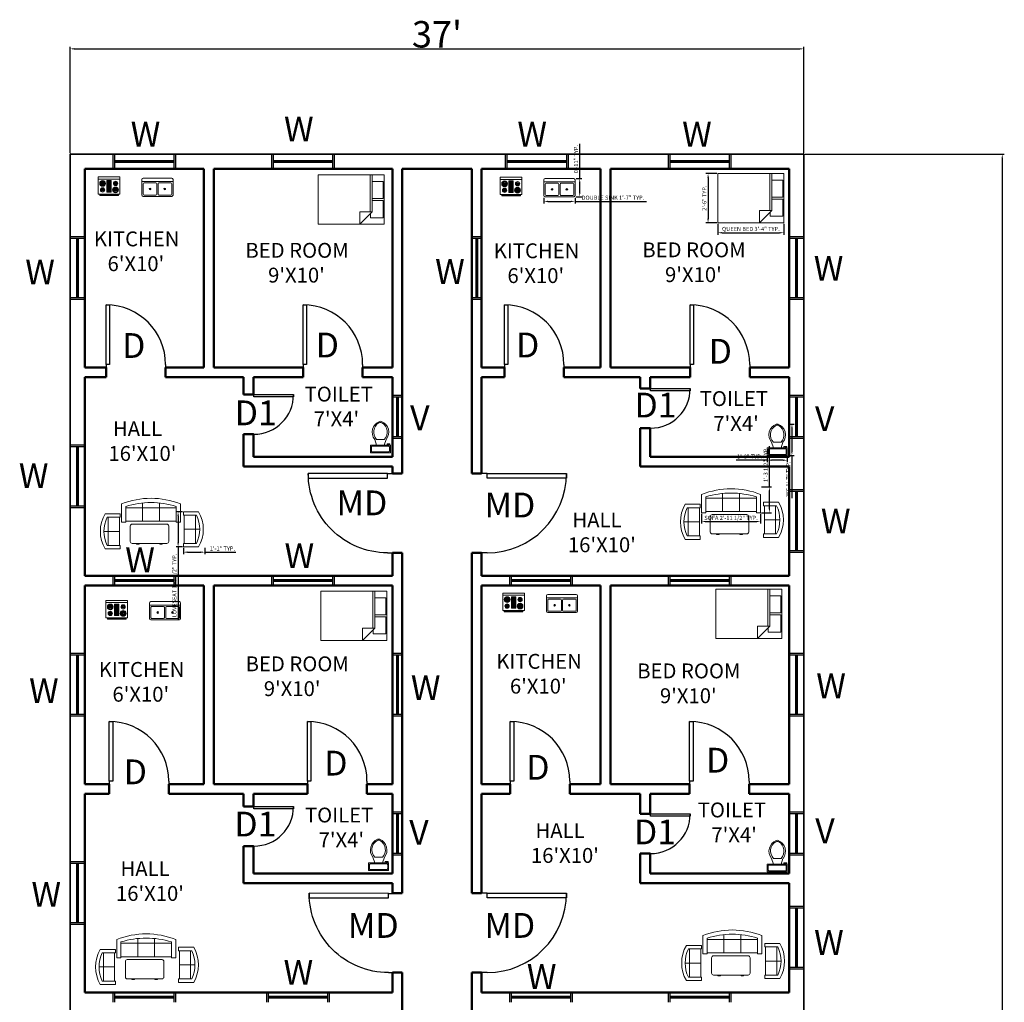
# Model space of a CAD drawing. Units: inches. Extents: x -25308 to -23933, y 10755 to 11996.
# Tile 6 of 6: x -24529 to -23933, y 11402 to 11996. Entities that reach past the tile are written whole.
import ezdxf

# ---------------------------------------------------------------- set-up
doc = ezdxf.new("R2010")
doc.units = ezdxf.units.IN
for name, color, linetype, lineweight in [('A-ANNO-DIMS', 2, 'Continuous', 18), ('A-ANNO-SYMB', 3, 'Continuous', 18), ('A-AREA-IDEN', 7, 'Continuous', 18), ('A-DOOR', 3, 'Continuous', 25), ('A-FLOR-FIXT', 8, 'Continuous', 18), ('A-FURN', 8, 'Continuous', 18), ('A-GLAZ', 4, 'Continuous', 25), ('A-WALL', 7, 'Continuous', 50), ('C-PROP', 30, 'Continuous', 35)]:
    doc.layers.add(name, color=color, linetype=linetype, lineweight=lineweight)
doc.styles.get("Standard").update_dxf_attribs({"font": 'arial.ttf'})
doc.dimstyles.new('ISO-25', dxfattribs={"dimtxt": 2.5, "dimasz": 2.5, "dimexe": 1.25, "dimexo": 0.625, "dimtad": 1, "dimdec": 0, "dimlunit": 3, "dimtxsty": 'Standard', "dimcen": 2.5, "dimadec": 0, "dimazin": 0, "dimtfac": 1, "dimtdec": 0, "dimtmove": 0, "dimatfit": 3, "dimfxl": 1, "dimarcsym": 0})

# ---------------------------------------------------------------- blocks, each defined once
blk = doc.blocks.new('*U8')
for p, q in [((0, 0), (0, -100)), ((750, 0), (750, -100))]:
    blk.add_line(p, q)
blk.add_lwpolyline([(0, 0), (0, 750), (43.75, 750), (43.75, 0)], close=True)
blk.add_arc((0, 0), 750, 0, 90)
blk = doc.blocks.new('Range-Oven - 30 in top')
for p, q in [((0, -3), (30, -3)), ((12, -6), (18, -6)), ((13, -20), (13, -6)), ((14, -6), (14, -20)), ((15, -20), (15, -6)), ((16, -6), (16, -20)), ((17, -20), (17, -6)), ((6, -24), (6, -25)), ((8, -25), (8, -24)), ((18, -20), (12, -20)), ((22, -25), (22, -24)), ((24, -24), (24, -25))]:
    blk.add_line(p, q)
for points in [[(0, -24), (0, 0), (30, 0), (30, -24)], [(12, -21), (12, -5), (18, -5), (18, -21)], [(2, -26), (2, -25), (28, -25), (28, -26)]]:
    blk.add_lwpolyline(points, close=True)
for centre, radius in [((6, -9), 4), ((6, -9), 3), ((6, -9), 2), ((6, -9), 1), ((24, -9), 3), ((24, -9), 2), ((24, -9), 1), ((6, -18), 3), ((6, -18), 2), ((6, -18), 1), ((24, -18), 4), ((24, -18), 3), ((24, -18), 2), ((24, -18), 1)]:
    blk.add_circle(centre, radius)
blk = doc.blocks.new('Sink-double - 36 in top')
for p, q in [((-18, -4), (18, -4)), ((-0.75, -18.5), (-0.75, -6.5)), ((0.75, -6.5), (0.75, -18.5))]:
    blk.add_line(p, q)
for points in [[(-16.5, 0), (16.5, 0)], [(-18, -19.5), (-18, -1.5)], [(-16.5, -18.5), (-16.5, -6.5)], [(-15.5, -5.5), (-1.75, -5.5)], [(1.75, -5.5), (15.5, -5.5)], [(16.5, -6.5), (16.5, -18.5)], [(18, -1.5), (18, -19.5)], [(16.5, -21), (-16.5, -21)], [(-1.75, -19.5), (-15.5, -19.5)], [(15.5, -19.5), (1.75, -19.5)]]:
    blk.add_lwpolyline(points)
for centre, radius in [((-8.5, -12.5), 1), ((-8.5, -12.5), 0.5), ((8.5, -12.5), 1), ((8.5, -12.5), 0.5)]:
    blk.add_circle(centre, radius)
for centre, radius, start, end in [((-16.5, -1.5), 1.5, 90, 180), ((16.5, -1.5), 1.5, 0, 90), ((-15.5, -6.5), 1, 90, 180), ((-1.75, -6.5), 1, 0, 90), ((1.75, -6.5), 1, 90, 180), ((15.5, -6.5), 1, 0, 90), ((-16.5, -19.5), 1.5, 180, 270), ((-15.5, -18.5), 1, 180, 270), ((-1.75, -18.5), 1, 270, 0), ((1.75, -18.5), 1, 180, 270), ((15.5, -18.5), 1, 270, 0), ((16.5, -19.5), 1.5, 270, 0)]:
    blk.add_arc(centre, radius, start, end)
blk = doc.blocks.new('Bed - Queen')
for p, q in [((0, -80.00003), (0, 0)), ((0, 0), (59.99999, 0)), ((59.99999, 0), (59.99999, -80.00003)), ((7.99999, -1.2), (28.79998, -1.2)), ((7.99999, -14.4), (7.99999, -1.2)), ((28.79998, -1.2), (28.79998, -14.4)), ((31.19999, -1.2), (51.99999, -1.2)), ((31.19999, -14.4), (31.19999, -1.2)), ((51.99999, -1.2), (51.99999, -16.4)), ((0, -14.4), (44.8, -14.4)), ((44.8, -16.8), (0, -16.8)), ((59.99999, -29.6), (44.8, -14.4)), ((44.8, -14.4), (44.8, -29.6)), ((51.99999, -16.4), (46.79936, -16.4)), ((44.8, -29.6), (59.99999, -29.6)), ((59.99999, -80.00003), (0, -80.00003))]:
    blk.add_line(p, q)
blk = doc.blocks.new('Desk - 30 x 60 in.')
for p, q in [((-26.999995, 0), (26.999995, 0)), ((-29.999995, -27), (-29.999995, -3)), ((29.999995, -3), (29.999995, -27)), ((26.999995, -30), (-26.999995, -30)), ((-20.000005, -30), (-20.000005, -31)), ((-16.000005, -31), (-16.000005, -30)), ((15.999995, -31), (15.999995, -30)), ((19.999995, -30), (19.999995, -31)), ((-20.000005, -31), (-16.000005, -31)), ((19.999995, -31), (15.999995, -31))]:
    blk.add_line(p, q)
for centre, start, end in [((-26.499995, -3.5), 98.1301, 171.8699), ((26.499995, -3.5), 8.130102, 81.8699), ((-26.499995, -26.5), 188.1301, 261.8699), ((26.499995, -26.5), 278.1301, 351.8699)]:
    blk.add_arc(centre, 3.535534, start, end)
blk = doc.blocks.new('Sofa - Roundback 7 ft.')
for p, q in [((-36.000027, -34), (-36.000027, -11.4696)), ((-35.999844, -13.3819), (35.9998, -13.3819)), ((-12.00002, -32.4421), (-12.00003, -6.5971)), ((11.99997, -32.4421), (11.99998, -6.5971)), ((35.99998, -34), (35.99998, -11.4696)), ((-36.000027, -32.4421), (35.99998, -32.4421))]:
    blk.add_line(p, q)
for points in [[(-36.000027, -34), (-42.000027, -34), (-42.000027, -8)], [(41.99998, -8), (41.99998, -34), (35.99998, -34)]]:
    blk.add_lwpolyline(points)
for centre, radius, start, end in [((0, -114.25), 114.25, 68.43141, 111.5686), ((-0.00001, -127.1968), 121.1968, 72.72033, 107.2797)]:
    blk.add_arc(centre, radius, start, end)
blk = doc.blocks.new('Sofa - Roundback Loveseat 5 ft.')
for p, q in [((-24, -33.99998), (-24, -11.46958)), ((-23.9998, -13.38178), (23.99986, -13.38178)), ((0, -32.44198), (0, -5.99998)), ((24.00004, -33.99998), (24.00004, -11.46958)), ((-24, -32.44198), (24.00004, -32.44198))]:
    blk.add_line(p, q)
for points in [[(-24, -33.99998), (-30, -33.99998), (-30, -7.99998)], [(30.00004, -7.99998), (30.00004, -33.99998), (24.00004, -33.99998)]]:
    blk.add_lwpolyline(points)
for centre, radius, start, end in [((0, -60.24998), 60.24998, 60.13715, 119.8628), ((0, -61.38438), 55.38444, 64.32083, 115.6792)]:
    blk.add_arc(centre, radius, start, end)
blk = doc.blocks.new('Toilet - top')
for p, q in [((-10, -8.5), (-8, -8.5)), ((-10, -9.5), (-10, -8.5)), ((-7, -9.5), (-10, -9.5)), ((-8, -8.5), (-8, -8)), ((-7, -8), (-7, -9.5)), ((-4, -8), (-6, -14)), ((4, -8), (6, -14)), ((9.5, -6), (9.5, -2)), ((4, -14), (-4, -14))]:
    blk.add_line(p, q)
blk.add_lwpolyline([(10.5, -8), (10.5, 0), (-10.5, 0), (-10.5, -8)], close=True)
for points in [[(-9.5, -2), (-9.5, -6)], [(8.5, -1), (-8.5, -1)], [(-8.5, -7), (8.5, -7)]]:
    blk.add_lwpolyline(points)
for centre, radius, start, end in [((-8.6, -1.9), 0.884, 81.8699, 188.1301), ((-8.6, -6.1), 0.884, 171.8699, 278.1301), ((8.6, -1.9), 0.884, 351.8699, 98.1301), ((8.6, -6.1), 0.884, 261.8699, 8.1301), ((3.5, -21.6), 12.2, 141.4691, 247.9714), ((4.2, -21.8), 11.3, 136.3677, 238.9468), ((-3.5, -21.6), 12.2, 292.0284, 38.5307), ((-4.2, -21.8), 11.3, 301.053, 43.6321), ((0, -27.9), 4, 245.7318, 294.2682), ((0, -29), 4, 254.8605, 285.1395)]:
    blk.add_arc(centre, radius, start, end)
blk = doc.blocks.new('*D172')
at = {"layer": 'A-ANNO-DIMS', "color": 0, "lineweight": -2, "transparency": 16777216}
for p, q in [((-24498.33, 11915.75), (-24498.33, 11980.03)), ((-24054.33, 11915.75), (-24054.33, 11980.03)), ((-24495.83, 11978.78), (-24056.83, 11978.78))]:
    blk.add_line(p, q, dxfattribs=at)
at = {"layer": 'A-ANNO-DIMS', "color": 0, "transparency": 16777216}
for points in [[(-24495.83, 11979.2), (-24495.83, 11978.37), (-24498.33, 11978.78)], [(-24056.83, 11979.2), (-24056.83, 11978.37), (-24054.33, 11978.78)]]:
    blk.add_solid(points, dxfattribs=at)
at = {"layer": 'Defpoints', "color": 0, "transparency": 16777216}
for p in [(-24054.33, 11978.78), (-24498.33, 11915.12), (-24054.33, 11915.12)]:
    blk.add_point(p, dxfattribs=at)
at = {"layer": 'A-ANNO-DIMS', "color": 0, "transparency": 16777216, "insert": (-24276.33, 11987.58), "char_height": 2.5, "attachment_point": 5}
blk.add_mtext("{\\H6.4x;37'}", dxfattribs=at)
blk = doc.blocks.new('*D173')
at = {"layer": 'A-ANNO-DIMS', "color": 0, "lineweight": -2, "transparency": 16777216}
for p, q in [((-24053.71, 11915.12), (-23933.08, 11915.12)), ((-23934.33, 11912.62), (-23934.33, 10813.62)), ((-24053.71, 10811.12), (-23933.08, 10811.12))]:
    blk.add_line(p, q, dxfattribs=at)
at = {"layer": 'A-ANNO-DIMS', "color": 0, "transparency": 16777216}
for points in [[(-23934.75, 11912.62), (-23933.91, 11912.62), (-23934.33, 11915.12)], [(-23934.75, 10813.62), (-23933.91, 10813.62), (-23934.33, 10811.12)]]:
    blk.add_solid(points, dxfattribs=at)
at = {"layer": 'Defpoints', "color": 0, "transparency": 16777216}
for p in [(-24054.33, 11915.12), (-24054.33, 10811.12), (-23934.33, 10811.12)]:
    blk.add_point(p, dxfattribs=at)
at = {"layer": 'A-ANNO-DIMS', "color": 0, "transparency": 16777216, "insert": (-23943.13, 11363.12), "char_height": 2.5, "attachment_point": 5, "rotation": 90}
blk.add_mtext("{\\H6.4x;92'}", dxfattribs=at)
blk = doc.blocks.new('WIN-36-9IN')
for p, q in [((0, 9), (0, 0)), ((1, 9), (1, 0)), ((37, 9), (37, 0)), ((38, 9), (38, 0)), ((1, 5), (37, 5)), ((1, 4.5), (37, 4.5)), ((1, 4), (37, 4))]:
    blk.add_line(p, q)
blk = doc.blocks.new('VENT-24')
for p, q in [((0, 26), (9, 26)), ((0, 25), (9, 25)), ((4, 1), (4, 25)), ((4.5, 1), (4.5, 25)), ((5, 1), (5, 25)), ((0, 1), (9, 1)), ((0, 0), (9, 0))]:
    blk.add_line(p, q)
blk = doc.blocks.new('WIN-24-6IN')
for p, q in [((0, 26), (6, 26)), ((0, 25), (6, 25)), ((2.5, 1), (2.5, 25)), ((3, 1), (3, 25)), ((3.5, 1), (3.5, 25)), ((0, 1), (6, 1)), ((0, 0), (6, 0))]:
    blk.add_line(p, q)
blk = doc.blocks.new('WIN-36-6IN')
for p, q in [((0, 6), (0, 0)), ((1, 6), (1, 0)), ((37, 6), (37, 0)), ((38, 6), (38, 0)), ((1, 3.5), (37, 3.5)), ((1, 3), (37, 3)), ((1, 2.5), (37, 2.5))]:
    blk.add_line(p, q)
blk = doc.blocks.new('*D194')
at = {"layer": 'A-ANNO-DIMS', "color": 0, "lineweight": -2, "transparency": 16777216}
for p, q in [((-24430.39, 11698.82), (-24434.2, 11698.82)), ((-24432.95, 11696.32), (-24432.95, 11680.06)), ((-24430.39, 11677.56), (-24434.2, 11677.56)), ((-24432.95, 11677.56), (-24432.95, 11633.45))]:
    blk.add_line(p, q, dxfattribs=at)
at = {"layer": 'A-ANNO-DIMS', "color": 0, "transparency": 16777216}
for points in [[(-24433.37, 11696.32), (-24432.53, 11696.32), (-24432.95, 11698.82)], [(-24433.37, 11680.06), (-24432.53, 11680.06), (-24432.95, 11677.56)]]:
    blk.add_solid(points, dxfattribs=at)
at = {"layer": 'Defpoints', "color": 0, "transparency": 16777216}
for p in [(-24429.76, 11698.82), (-24432.95, 11677.56), (-24429.76, 11677.56)]:
    blk.add_point(p, dxfattribs=at)
at = {"layer": 'A-ANNO-DIMS', "color": 0, "transparency": 16777216, "insert": (-24434.87, 11654.25), "char_height": 2.5, "attachment_point": 5, "rotation": 90}
blk.add_mtext('LOVESEAT 1\'-9 1/2" TYP.', dxfattribs=at)
blk = doc.blocks.new('*D195')
at = {"layer": 'A-ANNO-DIMS', "color": 0, "lineweight": -2, "transparency": 16777216}
for p, q in [((-24429.76, 11676.94), (-24429.76, 11673.12)), ((-24416.77, 11676.94), (-24416.77, 11673.12)), ((-24427.26, 11674.37), (-24419.27, 11674.37)), ((-24416.77, 11674.37), (-24398.02, 11674.37))]:
    blk.add_line(p, q, dxfattribs=at)
at = {"layer": 'A-ANNO-DIMS', "color": 0, "transparency": 16777216}
for points in [[(-24427.26, 11674.79), (-24427.26, 11673.95), (-24429.76, 11674.37)], [(-24419.27, 11674.79), (-24419.27, 11673.95), (-24416.77, 11674.37)]]:
    blk.add_solid(points, dxfattribs=at)
at = {"layer": 'Defpoints', "color": 0, "transparency": 16777216}
for p in [(-24429.76, 11677.56), (-24416.77, 11677.56), (-24416.77, 11674.37)]:
    blk.add_point(p, dxfattribs=at)
at = {"layer": 'A-ANNO-DIMS', "color": 0, "transparency": 16777216, "insert": (-24406.14, 11676.25), "char_height": 2.5, "attachment_point": 5}
blk.add_mtext('1\'-1" TYP.', dxfattribs=at)
blk = doc.blocks.new('*D200')
at = {"layer": 'A-ANNO-DIMS', "color": 0, "lineweight": -2, "transparency": 16777216}
for p, q in [((-24116.24, 11697.6), (-24116.24, 11691.62)), ((-24080.56, 11697.6), (-24080.56, 11691.62)), ((-24113.74, 11692.87), (-24083.06, 11692.87))]:
    blk.add_line(p, q, dxfattribs=at)
at = {"layer": 'A-ANNO-DIMS', "color": 0, "transparency": 16777216}
for points in [[(-24113.74, 11693.29), (-24113.74, 11692.45), (-24116.24, 11692.87)], [(-24083.06, 11693.29), (-24083.06, 11692.45), (-24080.56, 11692.87)]]:
    blk.add_solid(points, dxfattribs=at)
at = {"layer": 'Defpoints', "color": 0, "transparency": 16777216}
for p in [(-24116.24, 11698.22), (-24080.56, 11698.22), (-24080.56, 11692.87)]:
    blk.add_point(p, dxfattribs=at)
at = {"layer": 'A-ANNO-DIMS', "color": 0, "transparency": 16777216, "insert": (-24098.4, 11694.79), "char_height": 2.5, "attachment_point": 5}
blk.add_mtext('SOFA 2\'-11 1/2" TYP.', dxfattribs=at)
blk = doc.blocks.new('*D201')
at = {"layer": 'A-ANNO-DIMS', "color": 0, "lineweight": -2, "transparency": 16777216}
for p, q in [((-24075.2, 11713.8), (-24075.2, 11738.38)), ((-24079.93, 11713.8), (-24073.95, 11713.8)), ((-24075.2, 11700.72), (-24075.2, 11711.3)), ((-24079.93, 11698.22), (-24073.95, 11698.22))]:
    blk.add_line(p, q, dxfattribs=at)
at = {"layer": 'A-ANNO-DIMS', "color": 0, "transparency": 16777216}
for points in [[(-24075.62, 11711.3), (-24074.79, 11711.3), (-24075.2, 11713.8)], [(-24075.62, 11700.72), (-24074.79, 11700.72), (-24075.2, 11698.22)]]:
    blk.add_solid(points, dxfattribs=at)
at = {"layer": 'Defpoints', "color": 0, "transparency": 16777216}
for p in [(-24080.56, 11713.8), (-24075.2, 11713.8), (-24080.56, 11698.22)]:
    blk.add_point(p, dxfattribs=at)
at = {"layer": 'A-ANNO-DIMS', "color": 0, "transparency": 16777216, "insert": (-24077.12, 11727.34), "char_height": 2.5, "attachment_point": 5, "rotation": 90}
blk.add_mtext('1\'-3 1/2" TYP.', dxfattribs=at)
blk = doc.blocks.new('*D208')
at = {"layer": 'A-ANNO-DIMS', "color": 0, "lineweight": -2, "transparency": 16777216}
for p, q in [((-24106.34, 11872.9), (-24106.34, 11866.3)), ((-24066.52, 11872.9), (-24066.52, 11866.3)), ((-24103.84, 11867.55), (-24069.02, 11867.55))]:
    blk.add_line(p, q, dxfattribs=at)
at = {"layer": 'A-ANNO-DIMS', "color": 0, "transparency": 16777216}
for points in [[(-24103.84, 11867.97), (-24103.84, 11867.13), (-24106.34, 11867.55)], [(-24069.02, 11867.97), (-24069.02, 11867.13), (-24066.52, 11867.55)]]:
    blk.add_solid(points, dxfattribs=at)
at = {"layer": 'Defpoints', "color": 0, "transparency": 16777216}
for p in [(-24106.34, 11873.52), (-24066.52, 11873.52), (-24066.52, 11867.55)]:
    blk.add_point(p, dxfattribs=at)
at = {"layer": 'A-ANNO-DIMS', "color": 0, "transparency": 16777216, "insert": (-24086.43, 11869.54), "char_height": 2.5, "attachment_point": 5}
blk.add_mtext('QUEEN BED 3\'-4" TYP.', dxfattribs=at)
blk = doc.blocks.new('*D209')
at = {"layer": 'A-ANNO-DIMS', "color": 0, "lineweight": -2, "transparency": 16777216}
for p, q in [((-24106.97, 11903.39), (-24113.57, 11903.39)), ((-24112.32, 11900.89), (-24112.32, 11876.02)), ((-24106.97, 11873.52), (-24113.57, 11873.52))]:
    blk.add_line(p, q, dxfattribs=at)
at = {"layer": 'A-ANNO-DIMS', "color": 0, "transparency": 16777216}
for points in [[(-24112.73, 11900.89), (-24111.9, 11900.89), (-24112.32, 11903.39)], [(-24112.73, 11876.02), (-24111.9, 11876.02), (-24112.32, 11873.52)]]:
    blk.add_solid(points, dxfattribs=at)
at = {"layer": 'Defpoints', "color": 0, "transparency": 16777216}
for p in [(-24106.34, 11903.39), (-24112.32, 11873.52), (-24106.34, 11873.52)]:
    blk.add_point(p, dxfattribs=at)
at = {"layer": 'A-ANNO-DIMS', "color": 0, "transparency": 16777216, "insert": (-24114.22, 11888.46), "char_height": 2.5, "attachment_point": 5, "rotation": 90}
blk.add_mtext('2\'-6" TYP.', dxfattribs=at)
blk = doc.blocks.new('*D214')
at = {"layer": 'A-ANNO-DIMS', "color": 0, "lineweight": -2, "transparency": 16777216}
for p, q in [((-24063.8, 11751.85), (-24060.32, 11751.85)), ((-24061.57, 11749.35), (-24061.57, 11735.33)), ((-24063.8, 11732.83), (-24060.32, 11732.83)), ((-24061.57, 11732.83), (-24061.57, 11706.95))]:
    blk.add_line(p, q, dxfattribs=at)
at = {"layer": 'A-ANNO-DIMS', "color": 0, "transparency": 16777216}
for points in [[(-24061.99, 11749.35), (-24061.15, 11749.35), (-24061.57, 11751.85)], [(-24061.99, 11735.33), (-24061.15, 11735.33), (-24061.57, 11732.83)]]:
    blk.add_solid(points, dxfattribs=at)
at = {"layer": 'Defpoints', "color": 0, "transparency": 16777216}
for p in [(-24064.42, 11751.85), (-24064.42, 11732.83), (-24061.57, 11732.83)]:
    blk.add_point(p, dxfattribs=at)
at = {"layer": 'A-ANNO-DIMS', "color": 0, "transparency": 16777216, "insert": (-24063.49, 11718.64), "char_height": 2.5, "attachment_point": 5, "rotation": 90}
blk.add_mtext('WC 1\'-7" TYP.', dxfattribs=at)
blk = doc.blocks.new('*D215')
at = {"layer": 'A-ANNO-DIMS', "color": 0, "lineweight": -2, "transparency": 16777216}
for p, q in [((-24076.52, 11729.97), (-24095.27, 11729.97)), ((-24076.52, 11732.2), (-24076.52, 11728.72)), ((-24066.92, 11729.97), (-24074.02, 11729.97)), ((-24064.42, 11732.2), (-24064.42, 11728.72))]:
    blk.add_line(p, q, dxfattribs=at)
at = {"layer": 'A-ANNO-DIMS', "color": 0, "transparency": 16777216}
for points in [[(-24074.02, 11730.39), (-24074.02, 11729.56), (-24076.52, 11729.97)], [(-24066.92, 11730.39), (-24066.92, 11729.56), (-24064.42, 11729.97)]]:
    blk.add_solid(points, dxfattribs=at)
at = {"layer": 'Defpoints', "color": 0, "transparency": 16777216}
for p in [(-24076.52, 11732.83), (-24076.52, 11729.97), (-24064.42, 11732.83)]:
    blk.add_point(p, dxfattribs=at)
at = {"layer": 'A-ANNO-DIMS', "color": 0, "transparency": 16777216, "insert": (-24087.14, 11731.87), "char_height": 2.5, "attachment_point": 5}
blk.add_mtext('1\'-0" TYP.', dxfattribs=at)
blk = doc.blocks.new('*D218')
at = {"layer": 'A-ANNO-DIMS', "color": 0, "lineweight": -2, "transparency": 16777216}
for p, q in [((-24211.66, 11888.72), (-24211.66, 11885.27)), ((-24209.16, 11886.52), (-24195.3, 11886.52)), ((-24192.8, 11888.72), (-24192.8, 11885.27)), ((-24192.8, 11886.52), (-24149.48, 11886.52))]:
    blk.add_line(p, q, dxfattribs=at)
at = {"layer": 'A-ANNO-DIMS', "color": 0, "transparency": 16777216}
for points in [[(-24209.16, 11886.93), (-24209.16, 11886.1), (-24211.66, 11886.52)], [(-24195.3, 11886.93), (-24195.3, 11886.1), (-24192.8, 11886.52)]]:
    blk.add_solid(points, dxfattribs=at)
at = {"layer": 'Defpoints', "color": 0, "transparency": 16777216}
for p in [(-24211.66, 11889.35), (-24192.8, 11889.35), (-24192.8, 11886.52)]:
    blk.add_point(p, dxfattribs=at)
at = {"layer": 'A-ANNO-DIMS', "color": 0, "transparency": 16777216, "insert": (-24169.89, 11888.44), "char_height": 2.5, "attachment_point": 5}
blk.add_mtext('DOUBLE SINK 1\'-7" TYP.', dxfattribs=at)
blk = doc.blocks.new('*D219')
at = {"layer": 'A-ANNO-DIMS', "color": 0, "lineweight": -2, "transparency": 16777216}
for p, q in [((-24189.97, 11900.35), (-24189.97, 11921.28)), ((-24192.18, 11900.35), (-24188.72, 11900.35)), ((-24189.97, 11891.85), (-24189.97, 11897.85)), ((-24192.18, 11889.35), (-24188.72, 11889.35))]:
    blk.add_line(p, q, dxfattribs=at)
at = {"layer": 'A-ANNO-DIMS', "color": 0, "transparency": 16777216}
for points in [[(-24190.39, 11897.85), (-24189.56, 11897.85), (-24189.97, 11900.35)], [(-24190.39, 11891.85), (-24189.56, 11891.85), (-24189.97, 11889.35)]]:
    blk.add_solid(points, dxfattribs=at)
at = {"layer": 'Defpoints', "color": 0, "transparency": 16777216}
for p in [(-24192.8, 11900.35), (-24189.97, 11900.35), (-24192.8, 11889.35)]:
    blk.add_point(p, dxfattribs=at)
at = {"layer": 'A-ANNO-DIMS', "color": 0, "transparency": 16777216, "insert": (-24191.87, 11912.06), "char_height": 2.5, "attachment_point": 5, "rotation": 90}
blk.add_mtext('0\'-11" TYP.', dxfattribs=at)

msp = doc.modelspace()

# ---------------------------------------------------------------- linework, layer by layer
at = {"layer": 'A-WALL'}
for p, q in [((-24489.33, 11906.12), (-24417.33, 11906.12)), ((-24489.33, 11786.12), (-24489.33, 11906.12)), ((-24417.33, 11786.12), (-24417.33, 11906.12)), ((-24411.33, 11786.12), (-24411.33, 11906.12)), ((-24411.33, 11906.12), (-24303.33, 11906.12)), ((-24303.33, 11786.12), (-24303.33, 11906.12)), ((-24297.33, 11906.12), (-24255.33, 11906.12)), ((-24297.33, 11721.94), (-24297.33, 11906.12)), ((-24255.33, 11906.12), (-24255.33, 11721.94)), ((-24249.33, 11906.12), (-24249.33, 11786.12)), ((-24249.33, 11906.12), (-24177.33, 11906.12)), ((-24177.33, 11906.12), (-24177.33, 11786.12)), ((-24177.33, 11906.12), (-24177.33, 11786.12)), ((-24171.33, 11906.12), (-24171.33, 11786.12)), ((-24171.33, 11906.12), (-24171.33, 11786.12)), ((-24171.33, 11906.12), (-24063.33, 11906.12)), ((-24063.33, 11906.12), (-24063.33, 11786.12)), ((-24489.33, 11786.12), (-24476.55, 11786.12)), ((-24476.55, 11786.12), (-24476.55, 11780.12)), ((-24440.55, 11786.12), (-24440.55, 11780.12)), ((-24440.55, 11786.12), (-24417.33, 11786.12)), ((-24411.33, 11786.12), (-24357.3, 11786.12)), ((-24357.3, 11786.12), (-24357.3, 11780.12)), ((-24321.3, 11786.12), (-24321.3, 11780.12)), ((-24321.3, 11786.12), (-24303.33, 11786.12)), ((-24249.33, 11786.12), (-24235.5, 11786.12)), ((-24235.5, 11786.12), (-24235.5, 11780.12)), ((-24199.5, 11786.12), (-24199.5, 11780.12)), ((-24199.5, 11786.12), (-24177.33, 11786.12)), ((-24171.33, 11786.12), (-24123.14, 11786.12)), ((-24123.14, 11786.12), (-24123.14, 11780.12)), ((-24087.14, 11786.12), (-24087.14, 11780.12)), ((-24087.14, 11786.12), (-24063.33, 11786.12)), ((-24489.33, 11780.12), (-24476.55, 11780.12)), ((-24489.33, 11660.12), (-24489.33, 11780.12)), ((-24440.55, 11780.12), (-24393.33, 11780.12)), ((-24393.33, 11769.68), (-24393.33, 11780.12)), ((-24393.33, 11769.68), (-24393.33, 11780.12)), ((-24393.33, 11769.68), (-24393.33, 11780.12)), ((-24387.33, 11780.12), (-24357.3, 11780.12)), ((-24387.33, 11769.68), (-24387.33, 11780.12)), ((-24387.33, 11769.68), (-24387.33, 11780.12)), ((-24387.33, 11769.68), (-24387.33, 11780.12)), ((-24321.3, 11780.12), (-24303.33, 11780.12)), ((-24303.33, 11732.12), (-24303.33, 11780.12)), ((-24249.33, 11780.12), (-24235.5, 11780.12)), ((-24249.33, 11780.12), (-24249.33, 11721.94)), ((-24199.5, 11780.12), (-24153.33, 11780.12)), ((-24153.33, 11780.12), (-24153.33, 11773.35)), ((-24147.33, 11780.12), (-24147.33, 11773.35)), ((-24147.33, 11780.12), (-24123.14, 11780.12)), ((-24087.14, 11780.12), (-24063.33, 11780.12)), ((-24063.33, 11780.12), (-24063.33, 11732.12)), ((-24153.33, 11773.35), (-24147.33, 11773.35)), ((-24393.33, 11769.68), (-24387.33, 11769.68)), ((-24153.33, 11749.35), (-24147.33, 11749.35)), ((-24153.33, 11749.35), (-24153.33, 11726.12)), ((-24147.33, 11749.35), (-24147.33, 11732.12)), ((-24393.33, 11726.12), (-24393.33, 11745.68)), ((-24393.33, 11726.12), (-24393.33, 11745.68)), ((-24393.33, 11726.12), (-24393.33, 11745.68)), ((-24393.33, 11745.68), (-24387.33, 11745.68)), ((-24387.33, 11732.12), (-24387.33, 11745.68)), ((-24387.33, 11732.12), (-24387.33, 11745.68)), ((-24387.33, 11732.12), (-24387.33, 11745.68)), ((-24387.33, 11732.12), (-24303.33, 11732.12)), ((-24147.33, 11732.12), (-24063.33, 11732.12)), ((-24393.33, 11726.12), (-24303.33, 11726.12)), ((-24303.33, 11721.94), (-24303.33, 11726.12)), ((-24153.33, 11726.12), (-24063.33, 11726.12)), ((-24063.33, 11726.12), (-24063.33, 11660.12)), ((-24303.33, 11721.94), (-24297.33, 11721.94)), ((-24255.33, 11721.94), (-24249.33, 11721.94)), ((-24303.33, 11660.12), (-24303.33, 11673.94)), ((-24303.33, 11673.94), (-24297.33, 11673.94)), ((-24297.33, 11468.09), (-24297.33, 11673.94)), ((-24255.33, 11673.94), (-24249.33, 11673.94)), ((-24255.33, 11673.94), (-24255.33, 11468.09)), ((-24249.33, 11673.94), (-24249.33, 11660.12)), ((-24489.33, 11660.12), (-24303.33, 11660.12)), ((-24249.33, 11660.12), (-24063.33, 11660.12)), ((-24489.33, 11654.12), (-24417.33, 11654.12)), ((-24489.33, 11534.12), (-24489.33, 11654.12)), ((-24417.33, 11534.12), (-24417.33, 11654.12)), ((-24411.33, 11534.12), (-24411.33, 11654.12)), ((-24411.33, 11654.12), (-24303.33, 11654.12)), ((-24303.33, 11534.12), (-24303.33, 11654.12)), ((-24249.33, 11654.12), (-24177.33, 11654.12)), ((-24249.33, 11654.12), (-24249.33, 11534.12)), ((-24177.33, 11654.12), (-24177.33, 11534.12)), ((-24171.33, 11654.12), (-24171.33, 11534.12)), ((-24171.33, 11654.12), (-24063.33, 11654.12)), ((-24063.33, 11654.12), (-24063.33, 11534.12)), ((-24489.33, 11534.12), (-24474.63, 11534.12)), ((-24474.63, 11534.12), (-24474.63, 11528.12)), ((-24438.63, 11534.12), (-24438.63, 11528.12)), ((-24438.63, 11534.12), (-24417.33, 11534.12)), ((-24411.33, 11534.12), (-24354.67, 11534.12)), ((-24354.67, 11534.12), (-24354.67, 11528.12)), ((-24318.67, 11534.12), (-24318.67, 11528.12)), ((-24318.67, 11534.12), (-24303.33, 11534.12)), ((-24249.33, 11534.12), (-24231.97, 11534.12)), ((-24231.97, 11534.12), (-24231.97, 11528.12)), ((-24195.97, 11534.12), (-24195.97, 11528.12)), ((-24195.97, 11534.12), (-24177.33, 11534.12)), ((-24171.33, 11534.12), (-24123.45, 11534.12)), ((-24123.45, 11534.12), (-24123.45, 11528.12)), ((-24087.45, 11534.12), (-24087.45, 11528.12)), ((-24087.45, 11534.12), (-24063.33, 11534.12)), ((-24489.33, 11528.12), (-24474.63, 11528.12)), ((-24489.33, 11408.12), (-24489.33, 11528.12)), ((-24438.63, 11528.12), (-24393.33, 11528.12)), ((-24393.33, 11520.57), (-24393.33, 11528.12)), ((-24393.33, 11520.57), (-24393.33, 11528.12)), ((-24387.33, 11528.12), (-24354.67, 11528.12)), ((-24387.33, 11520.57), (-24387.33, 11528.12)), ((-24387.33, 11520.57), (-24387.33, 11528.12)), ((-24318.67, 11528.12), (-24303.33, 11528.12)), ((-24303.33, 11480.12), (-24303.33, 11528.12)), ((-24249.33, 11528.12), (-24231.97, 11528.12)), ((-24249.33, 11528.12), (-24249.33, 11468.09)), ((-24195.97, 11528.12), (-24153.33, 11528.12)), ((-24153.33, 11528.12), (-24153.33, 11516.06)), ((-24147.33, 11528.12), (-24147.33, 11516.06)), ((-24147.33, 11528.12), (-24123.45, 11528.12)), ((-24087.45, 11528.12), (-24063.33, 11528.12)), ((-24063.33, 11528.12), (-24063.33, 11480.12)), ((-24393.33, 11520.57), (-24387.33, 11520.57)), ((-24153.33, 11516.06), (-24147.33, 11516.06)), ((-24393.33, 11474.12), (-24393.33, 11496.57)), ((-24393.33, 11474.12), (-24393.33, 11496.57)), ((-24393.33, 11496.57), (-24387.33, 11496.57)), ((-24387.33, 11480.12), (-24387.33, 11496.57)), ((-24387.33, 11480.12), (-24387.33, 11496.57)), ((-24153.33, 11492.06), (-24147.33, 11492.06)), ((-24153.33, 11492.06), (-24153.33, 11474.12)), ((-24147.33, 11492.06), (-24147.33, 11480.12)), ((-24387.33, 11480.12), (-24303.33, 11480.12)), ((-24147.33, 11480.12), (-24063.33, 11480.12)), ((-24393.33, 11474.12), (-24303.33, 11474.12)), ((-24303.33, 11468.09), (-24303.33, 11474.12)), ((-24153.33, 11474.12), (-24063.33, 11474.12)), ((-24063.33, 11474.12), (-24063.33, 11408.12)), ((-24303.33, 11468.09), (-24297.33, 11468.09)), ((-24255.33, 11468.09), (-24249.33, 11468.09)), ((-24303.33, 11408.12), (-24303.33, 11420.09)), ((-24303.33, 11420.09), (-24297.33, 11420.09)), ((-24297.33, 11211.71), (-24297.33, 11420.09)), ((-24255.33, 11420.09), (-24249.33, 11420.09)), ((-24255.33, 11420.09), (-24255.33, 11211.71)), ((-24249.33, 11420.09), (-24249.33, 11408.12)), ((-24489.33, 11408.12), (-24387.33, 11408.12)), ((-24387.33, 11408.12), (-24303.33, 11408.12)), ((-24249.33, 11408.12), (-24063.33, 11408.12))]:
    msp.add_line(p, q, dxfattribs=at)
at = {"layer": 'C-PROP'}
for p, q in [((-24498.33, 11915.12), (-24054.33, 11915.12)), ((-24498.33, 10811.12), (-24498.33, 11915.12)), ((-24054.33, 11915.12), (-24054.33, 10811.12))]:
    msp.add_line(p, q, dxfattribs=at)

# ---------------------------------------------------------------- block references
at = {"layer": 'A-DOOR', "xscale": 0.0480000000000013, "yscale": 0.0480000000000013, "zscale": 0.0480000000000013}
for p in [(-24476.55, 11787.92), (-24357.3, 11787.92), (-24235.5, 11787.92), (-24123.14, 11787.92), (-24474.63, 11535.92), (-24354.67, 11535.92), (-24231.97, 11535.92), (-24123.45, 11535.92)]:
    msp.add_blockref('*U8', p, dxfattribs=at)
at = {"layer": 'A-DOOR'}
for p, xscale, yscale, zscale, rotation in [((-24147.13, 11773.35), 0.0320000053173207, 0.0320000053173207, 0.0320000053173207, 270.0087240591115), ((-24387.13, 11769.68), 0.0320000053173207, 0.0320000053173207, 0.0320000053173207, 270.0087240591115), ((-24306.26, 11721.91), -0.0639171163268206, 0.0639171163268206, 0.0639171163268206, 89.99127594088849), ((-24245.94, 11721.94), 0.064000001883637, 0.064000001883637, 0.064000001883637, 270.0087240591115), ((-24387.13, 11520.57), 0.0320000053173207, 0.0320000053173207, 0.0320000053173207, 270.0087240591115), ((-24147.13, 11516.06), 0.0320000053173207, 0.0320000053173207, 0.0320000053173207, 270.0087240591115), ((-24305.72, 11468.02), -0.0639171163268206, 0.0639171163268206, 0.0639171163268206, 89.99127594088849), ((-24245.93, 11468.1), 0.064000001883637, 0.064000001883637, 0.064000001883637, 270.0087240591115)]:
    msp.add_blockref('*U8', p, dxfattribs=dict(at, xscale=xscale, yscale=yscale, zscale=zscale, rotation=rotation))
at = {"layer": 'A-FLOR-FIXT'}
for name, p, xscale, yscale, zscale in [('Range-Oven - 30 in top', (-24481.25, 11901.31), 0.4346134936801813, 0.4346134936801813, 0.4346134936801813), ('Sink-double - 36 in top', (-24445.46, 11900.57), 0.5237879159203632, 0.5237879159203632, 0.5237879159203632), ('Range-Oven - 30 in top', (-24238.02, 11901.09), 0.4346134936801813, 0.4346134936801813, 0.4346134936801813), ('Sink-double - 36 in top', (-24202.23, 11900.35), 0.5237879159203632, 0.5237879159203632, 0.5237879159203632), ('Range-Oven - 30 in top', (-24236.48, 11649.58), 0.4346134936801813, 0.4346134936801813, 0.4346134936801813), ('Sink-double - 36 in top', (-24200.69, 11648.83), 0.5237879159203632, 0.5237879159203632, 0.5237879159203632), ('Range-Oven - 30 in top', (-24476.62, 11645.18), 0.4346134936801813, 0.4346134936801813, 0.4346134936801813), ('Sink-double - 36 in top', (-24440.83, 11644.43), 0.5237879159203632, 0.5237879159203632, 0.5237879159203632)]:
    msp.add_blockref(name, p, dxfattribs=dict(at, xscale=xscale, yscale=yscale, zscale=zscale))
at = {"layer": 'A-FLOR-FIXT', "xscale": 0.5757571651567317, "yscale": 0.5757571651567317, "zscale": 0.5757571651567317, "rotation": 180}
for p in [(-24310.53, 11734.5), (-24070.47, 11732.83), (-24311.62, 11481.78), (-24070.45, 11481.09)]:
    msp.add_blockref('Toilet - top', p, dxfattribs=at)
at = {"layer": 'A-FURN'}
for name, p, xscale, yscale, zscale, rotation in [('Bed - Queen', (-24308.36, 11902.54), 0.4977730924347652, 0.4977730924347652, 0.4977730924347652, 270), ('Bed - Queen', (-24066.52, 11903.39), 0.4977730924347652, 0.4977730924347652, 0.4977730924347652, 270), ('Sofa - Roundback Loveseat 5 ft.', (-24129.04, 11692.67), 0.3543289087725223, 0.3543289087725223, 0.3543289087725223, 89.99999999999999), ('Sofa - Roundback Loveseat 5 ft.', (-24066.77, 11693.92), 0.3543289087725223, 0.3543289087725223, 0.3543289087725223, 270), ('Sofa - Roundback Loveseat 5 ft.', (-24479.98, 11686.94), 0.3543289087725223, 0.3543289087725223, 0.3543289087725223, 89.99999999999999), ('Sofa - Roundback Loveseat 5 ft.', (-24417.71, 11688.19), 0.3543289087725223, 0.3543289087725223, 0.3543289087725223, 270), ('Bed - Queen', (-24306.68, 11650.78), 0.4977730924347652, 0.4977730924347652, 0.4977730924347652, 270), ('Bed - Queen', (-24067.71, 11651.93), 0.4977730924347652, 0.4977730924347652, 0.4977730924347652, 270), ('Sofa - Roundback Loveseat 5 ft.', (-24066.01, 11427.1), 0.3543289087725223, 0.3543289087725223, 0.3543289087725223, 270), ('Sofa - Roundback Loveseat 5 ft.', (-24482.89, 11423.5), 0.3543289087725223, 0.3543289087725223, 0.3543289087725223, 89.99999999999999), ('Sofa - Roundback Loveseat 5 ft.', (-24420.62, 11424.75), 0.3543289087725223, 0.3543289087725223, 0.3543289087725223, 270), ('Sofa - Roundback Loveseat 5 ft.', (-24128.28, 11425.86), 0.3543289087725223, 0.3543289087725223, 0.3543289087725223, 89.99999999999999)]:
    msp.add_blockref(name, p, dxfattribs=dict(at, xscale=xscale, yscale=yscale, zscale=zscale, rotation=rotation))
for name, p, xscale, yscale, zscale in [('Sofa - Roundback 7 ft.', (-24098.4, 11712.67), 0.4248490443916877, 0.4248490443916877, 0.4248490443916877), ('Sofa - Roundback 7 ft.', (-24449.34, 11706.94), 0.4248490443916877, 0.4248490443916877, 0.4248490443916877), ('Desk - 30 x 60 in.', (-24099.35, 11697.08), 0.3893791270499034, 0.3893791270499034, 0.3893791270499034), ('Desk - 30 x 60 in.', (-24450.29, 11691.35), 0.3893791270499034, 0.3893791270499034, 0.3893791270499034), ('Sofa - Roundback 7 ft.', (-24452.25, 11443.5), 0.4248490443916877, 0.4248490443916877, 0.4248490443916877), ('Sofa - Roundback 7 ft.', (-24097.64, 11445.85), 0.4248490443916877, 0.4248490443916877, 0.4248490443916877), ('Desk - 30 x 60 in.', (-24453.19, 11427.91), 0.3893791270499034, 0.3893791270499034, 0.3893791270499034), ('Desk - 30 x 60 in.', (-24098.58, 11430.26), 0.3893791270499034, 0.3893791270499034, 0.3893791270499034)]:
    msp.add_blockref(name, p, dxfattribs=dict(at, xscale=xscale, yscale=yscale, zscale=zscale))
at = {"layer": 'A-GLAZ'}
for name, p, rotation in [('WIN-36-9IN', (-24434.33, 11915.12), 180), ('WIN-36-9IN', (-24434.33, 11915.12), 180), ('WIN-36-9IN', (-24338.33, 11915.12), 180), ('WIN-36-9IN', (-24338.33, 11915.12), 180), ('WIN-36-9IN', (-24196.78, 11915.12), 180), ('WIN-36-9IN', (-24196.78, 11915.12), 180), ('WIN-36-9IN', (-24098.33, 11915.12), 180), ('WIN-36-9IN', (-24498.33, 11865.12), 270.0000000000211), ('WIN-36-6IN', (-24255.33, 11865.12), 270.0000000000143), ('WIN-36-9IN', (-24063.33, 11865.12), 270.0000000000211), ('WIN-24-6IN', (-24297.33, 11769.12), 180), ('VENT-24', (-24054.33, 11769.12), 180), ('WIN-36-9IN', (-24498.33, 11739.12), 270.0000000000211), ('WIN-36-9IN', (-24063.33, 11712.12), 270.0000000000173), ('WIN-36-6IN', (-24434.33, 11660.12), 180), ('WIN-36-6IN', (-24338.33, 11660.12), 180), ('WIN-36-6IN', (-24194.33, 11660.12), 180), ('WIN-36-6IN', (-24098.33, 11660.12), 180), ('WIN-36-9IN', (-24498.33, 11613.12), 270.0000000000443), ('WIN-36-6IN', (-24303.33, 11613.12), 270.0000000000161), ('WIN-36-9IN', (-24063.33, 11613.12), 270.0000000000235), ('WIN-24-6IN', (-24297.33, 11517.12), 180), ('VENT-24', (-24054.33, 11517.12), 180), ('WIN-36-9IN', (-24498.33, 11487.12), 270.0000000000211), ('WIN-36-9IN', (-24063.33, 11460.12), 270.0000000000211), ('WIN-36-6IN', (-24434.33, 11408.12), 180), ('WIN-36-6IN', (-24341.33, 11408.12), 180), ('WIN-36-6IN', (-24194.33, 11408.12), 180), ('WIN-36-6IN', (-24098.33, 11408.12), 180)]:
    msp.add_blockref(name, p, dxfattribs=dict(at, rotation=rotation))

# ---------------------------------------------------------------- texts
at = {"layer": 'A-ANNO-SYMB', "char_height": 15, "attachment_point": 1}
for s, insert in [('{W}', (-24461.65, 11934.71)), ('{W}', (-24368.9, 11937.77)), ('{W}', (-24227.72, 11934.71)), ('{W}', (-24128, 11934.71)), ('{W}', (-24525.45, 11851.33)), ('{W}', (-24277.45, 11851.65)), ('{W}', (-24048.37, 11853.56)), ('{D}', (-24349.7, 11807.13)), ('{D}', (-24228.5, 11807.16)), ('{D}', (-24466.84, 11806.84)), ('{D}', (-24111.95, 11803.35)), ('{D1}', (-24398.7, 11766.11)), ('{D1}', (-24156.82, 11770.82)), ('{V}', (-24292.59, 11763.11)), ('{V}', (-24047.64, 11762.66)), ('{W}', (-24529.32, 11728.15)), ('{MD}', (-24337.08, 11711.67)), ('{MD}', (-24247.54, 11710.36)), ('{W}', (-24044.05, 11700.67)), ('{W}', (-24464.96, 11677.21)), ('{W}', (-24368.57, 11679.71)), ('{W}', (-24292.15, 11599.94)), ('{W}', (-24046.88, 11601.03)), ('{W}', (-24523.13, 11598.14)), ('{D}', (-24344.52, 11554.27)), ('{D}', (-24222.29, 11551.74)), ('{D}', (-24113.56, 11556.05)), ('{D}', (-24465.87, 11548.99)), ('{D1}', (-24398.92, 11517.4)), ('{V}', (-24293.13, 11512.41)), ('{D1}', (-24157.14, 11512.66)), ('{V}', (-24047.46, 11513.33)), ('{W}', (-24521.71, 11474.96)), ('{MD}', (-24330.2, 11456.11)), ('{MD}', (-24247.61, 11456.11)), ('{W}', (-24048.17, 11445.82)), ('{W}', (-24369.16, 11427.71)), ('{W}', (-24221.97, 11425.21))]:
    msp.add_mtext_dynamic_manual_height_columns(s, width=853.3083, gutter_width=12.5, heights=[0], dxfattribs=dict(at, insert=insert))
at = {"layer": 'A-AREA-IDEN', "char_height": 9, "attachment_point": 1}
for s, insert in [("{KITCHEN\\P   6'X10'}", (-24483.9, 11868.34)), ("{BED ROOM\\P     9'X10'}", (-24392.24, 11861.42)), ("{KITCHEN\\P   6'X10'}", (-24241.96, 11861.14)), ("{BED ROOM\\P     9'X10'}", (-24152.09, 11861.72)), ("{  TOILET\\P    7'X4'}", (-24361.92, 11774.46)), ("{  TOILET\\P     7'X4'}", (-24122.87, 11771.75)), ("{ HALL\\P16'X10'}", (-24475.12, 11753.57)), ("{ HALL\\P16'X10'}", (-24197.12, 11698.35)), ("{BED ROOM\\P    9'X10'}", (-24392.11, 11611.33)), ("{KITCHEN\\P   6'X10'}", (-24240.44, 11612.84)), ("{KITCHEN\\P   6'X10'}", (-24480.93, 11607.94)), ("{BED ROOM\\P     9'X10'}", (-24155.18, 11607.04)), ("{     TOILET\\P        7'X4'}", (-24132.3, 11522.95)), ("{  TOILET\\P     7'X4'}", (-24361.69, 11519.88)), ("{        HALL\\P       16'X10'}", (-24238.73, 11510.45)), ("{    HALL \\P   16'X10'}", (-24478.8, 11487.46))]:
    msp.add_mtext_dynamic_manual_height_columns(s, width=853.3083, gutter_width=12.5, heights=[0], dxfattribs=dict(at, insert=insert))

# ---------------------------------------------------------------- dimensions: what is measured, and where the dimension line sits
at = {"layer": 'A-ANNO-DIMS'}
for base, p1, p2, text, override, picture, middle in [((-24054.33, 11978.78), (-24498.33, 11915.12), (-24054.33, 11915.12), '{\\H6.4x;<>}', {"dimclrd": 0, "dimclre": 0, "dimclrt": 0}, '*D172', (-24276.33, 11987.58)), ((-24192.8, 11886.52), (-24211.66, 11889.35), (-24192.8, 11889.35), 'DOUBLE SINK <> TYP.', {"dimdec": 1, "dimlfac": 1, "dimrnd": 0, "dimzin": 1, "dimdsep": 46, "dimlunit": 4, "dimfrac": 2}, '*D218', (-24169.89, 11888.44)), ((-24066.52, 11867.55), (-24106.34, 11873.52), (-24066.52, 11873.52), 'QUEEN BED <> TYP.', {"dimdec": 1, "dimlfac": 1, "dimrnd": 0, "dimzin": 1, "dimdsep": 46, "dimlunit": 4, "dimfrac": 2}, '*D208', (-24086.43, 11869.54)), ((-24080.56, 11692.87), (-24116.24, 11698.22), (-24080.56, 11698.22), 'SOFA <> TYP.', {"dimdec": 1, "dimlfac": 1, "dimrnd": 0, "dimzin": 1, "dimdsep": 46, "dimlunit": 4, "dimfrac": 2}, '*D200', (-24098.4, 11694.79)), ((-24416.77, 11674.37), (-24429.76, 11677.56), (-24416.77, 11677.56), '<> TYP.', {"dimdec": 1, "dimlfac": 1, "dimrnd": 0, "dimzin": 1, "dimdsep": 46, "dimlunit": 4, "dimfrac": 2}, '*D195', (-24406.14, 11676.25))]:
    dim = msp.add_linear_dim(base=base, p1=p1, p2=p2, text=text, dimstyle='ISO-25', override=override, dxfattribs=at)
    dim.commit()
    dim.dimension.update_dxf_attribs({"geometry": picture, "text_midpoint": middle})
for base, p1, p2, angle, text, override, picture, middle in [((-24189.97, 11900.35), (-24192.8, 11889.35), (-24192.8, 11900.35), 90, '<> TYP.', {"dimdec": 1, "dimlfac": 1, "dimrnd": 0, "dimzin": 1, "dimdsep": 46, "dimlunit": 4, "dimfrac": 2}, '*D219', (-24191.87, 11912.06)), ((-23934.33, 10811.12), (-24054.33, 11915.12), (-24054.33, 10811.12), 90, '{\\H6.4x;<>}', {"dimclrd": 0, "dimclre": 0, "dimclrt": 0}, '*D173', (-23943.13, 11363.12)), ((-24112.32, 11873.52), (-24106.34, 11903.39), (-24106.34, 11873.52), 270, '<> TYP.', {"dimdec": 1, "dimlfac": 1, "dimrnd": 0, "dimzin": 1, "dimdsep": 46, "dimlunit": 4, "dimfrac": 2}, '*D209', (-24114.22, 11888.46)), ((-24061.57, 11732.83), (-24064.42, 11751.85), (-24064.42, 11732.83), 270, 'WC <> TYP.', {"dimdec": 1, "dimlfac": 1, "dimrnd": 0, "dimzin": 1, "dimdsep": 46, "dimlunit": 4, "dimfrac": 2}, '*D214', (-24063.49, 11718.64)), ((-24076.52, 11729.97), (-24064.42, 11732.83), (-24076.52, 11732.83), 180, '<> TYP.', {"dimdec": 1, "dimlfac": 1, "dimrnd": 0, "dimzin": 1, "dimdsep": 46, "dimlunit": 4, "dimfrac": 2}, '*D215', (-24087.14, 11731.87)), ((-24075.2, 11713.8), (-24080.56, 11698.22), (-24080.56, 11713.8), 90, '<> TYP.', {"dimdec": 1, "dimlfac": 1, "dimrnd": 0, "dimzin": 1, "dimdsep": 46, "dimlunit": 4, "dimfrac": 2}, '*D201', (-24077.12, 11727.34)), ((-24432.95, 11677.56), (-24429.76, 11698.82), (-24429.76, 11677.56), 270, 'LOVESEAT <> TYP.', {"dimdec": 1, "dimlfac": 1, "dimrnd": 0, "dimzin": 1, "dimdsep": 46, "dimlunit": 4, "dimfrac": 2}, '*D194', (-24434.87, 11654.25))]:
    dim = msp.add_linear_dim(base=base, p1=p1, p2=p2, angle=angle, text=text, dimstyle='ISO-25', override=override, dxfattribs=at)
    dim.commit()
    dim.dimension.update_dxf_attribs({"geometry": picture, "text_midpoint": middle})

doc.saveas('drawing.dxf')
